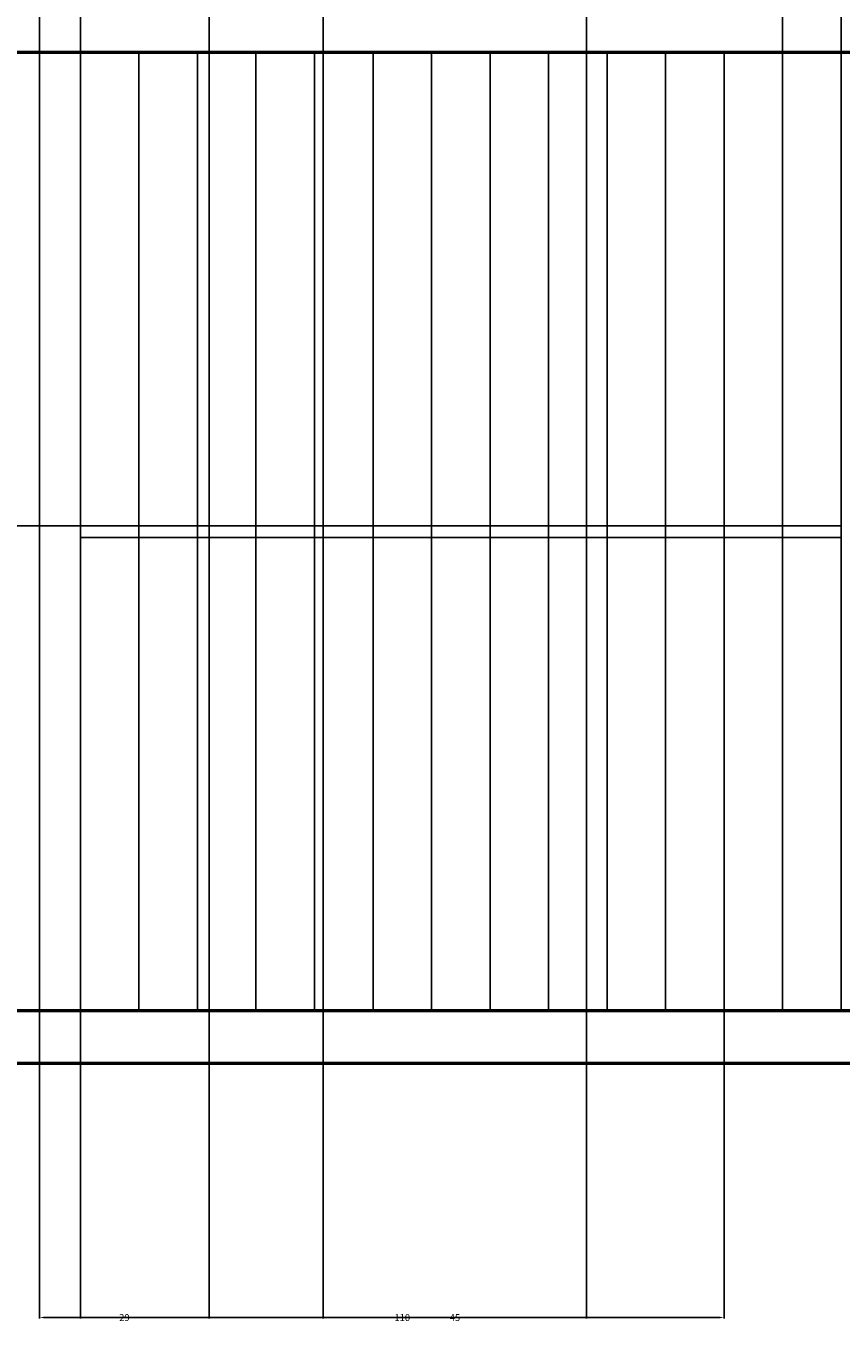
# Model space of a CAD drawing. Units: inches. Extents: x 3506 to 3958, y 1553 to 2506.
# Tile 2 of 16: x 3599 to 3739, y 1553 to 1775. Entities that reach past the tile are written whole.
import ezdxf

# ---------------------------------------------------------------- set-up
doc = ezdxf.new("R2010")
doc.units = ezdxf.units.IN
doc.header["$MEASUREMENT"] = 0
for name, color, linetype, lineweight in [('A-ANNO-DIMS', 2, 'Continuous', 18), ('A-FLOR-STRS', 7, 'Continuous', 25), ('A-WALL', 7, 'Continuous', 50)]:
    doc.layers.add(name, color=color, linetype=linetype, lineweight=lineweight)
doc.layers.add('A-WALL-PATT', color=251, linetype='Continuous', lineweight=13, true_color=0x636466)
doc.styles.get("Standard").update_dxf_attribs({"font": 'arial.ttf'})
doc.dimstyles.get("Standard").update_dxf_attribs({"dimtxt": 1.18, "dimasz": 0.68, "dimexe": 0.18, "dimexo": 0.0625, "dimgap": 0.09, "dimtad": 0, "dimtih": 1, "dimtoh": 1, "dimdec": 1, "dimzin": 0, "dimdsep": 46, "dimlunit": 3, "dimtxsty": 'Standard', "dimcen": 0.09, "dimadec": 0, "dimazin": 0, "dimtfac": 1, "dimtdec": 1, "dimtofl": 0, "dimtmove": 0, "dimatfit": 3, "dimfxl": 1, "dimtolj": 1, "dimtzin": 0, "dimarcsym": 0})

# ---------------------------------------------------------------- blocks, each defined once
blk = doc.blocks.new('*D50')
at = {"layer": 'A-ANNO-DIMS', "color": 0, "lineweight": -2, "transparency": 16777216}
for p, q in [((3608.73, 1606.46), (3608.73, 2505.02)), ((3609.41, 2504.84), (3672.39, 2504.84)), ((3738.05, 2504.84), (3675.07, 2504.84)), ((3738.73, 1606.46), (3738.73, 2505.02))]:
    blk.add_line(p, q, dxfattribs=at)
at = {"layer": 'A-ANNO-DIMS', "color": 0, "transparency": 16777216}
for points in [[(3609.41, 2504.96), (3609.41, 2504.73), (3608.73, 2504.84)], [(3738.05, 2504.96), (3738.05, 2504.73), (3738.73, 2504.84)]]:
    blk.add_solid(points, dxfattribs=at)
at = {"layer": 'Defpoints', "color": 0, "transparency": 16777216}
for p in [(3738.73, 2504.84), (3608.73, 1606.39), (3738.73, 1606.39)]:
    blk.add_point(p, dxfattribs=at)
at = {"layer": 'A-ANNO-DIMS', "color": 0, "transparency": 16777216, "insert": (3673.73, 2504.84), "char_height": 1.18, "attachment_point": 5}
blk.add_mtext('\\A1;130', dxfattribs=at)
blk = doc.blocks.new('*D51')
at = {"layer": 'A-ANNO-DIMS', "color": 0, "lineweight": -2, "transparency": 16777216}
for p, q in [((3608.67, 1689.39), (3508.1, 1689.39)), ((3508.28, 1688.71), (3508.28, 1648.59)), ((3508.28, 1607.07), (3508.28, 1647.2)), ((3608.67, 1606.39), (3508.1, 1606.39))]:
    blk.add_line(p, q, dxfattribs=at)
at = {"layer": 'A-ANNO-DIMS', "color": 0, "transparency": 16777216}
for points in [[(3508.17, 1688.71), (3508.39, 1688.71), (3508.28, 1689.39)], [(3508.17, 1607.07), (3508.39, 1607.07), (3508.28, 1606.39)]]:
    blk.add_solid(points, dxfattribs=at)
at = {"layer": 'Defpoints', "color": 0, "transparency": 16777216}
for p in [(3508.28, 1689.39), (3608.73, 1689.39), (3608.73, 1606.39)]:
    blk.add_point(p, dxfattribs=at)
at = {"layer": 'A-ANNO-DIMS', "color": 0, "transparency": 16777216, "insert": (3508.28, 1647.89), "char_height": 1.18, "attachment_point": 5}
blk.add_mtext('\\A1;83', dxfattribs=at)
blk = doc.blocks.new('*D52')
at = {"layer": 'A-ANNO-DIMS', "color": 0, "lineweight": -2, "transparency": 16777216}
for p, q in [((3560.73, 1606.46), (3560.73, 2505.02)), ((3561.41, 2504.84), (3583.77, 2504.84)), ((3608.05, 2504.84), (3585.69, 2504.84)), ((3608.73, 1606.46), (3608.73, 2505.02))]:
    blk.add_line(p, q, dxfattribs=at)
at = {"layer": 'A-ANNO-DIMS', "color": 0, "transparency": 16777216}
for points in [[(3561.41, 2504.96), (3561.41, 2504.73), (3560.73, 2504.84)], [(3608.05, 2504.96), (3608.05, 2504.73), (3608.73, 2504.84)]]:
    blk.add_solid(points, dxfattribs=at)
at = {"layer": 'Defpoints', "color": 0, "transparency": 16777216}
for p in [(3608.73, 2504.84), (3560.73, 1606.39), (3608.73, 1606.39)]:
    blk.add_point(p, dxfattribs=at)
at = {"layer": 'A-ANNO-DIMS', "color": 0, "transparency": 16777216, "insert": (3584.73, 2504.84), "char_height": 1.18, "attachment_point": 5}
blk.add_mtext('\\A1;48', dxfattribs=at)
blk = doc.blocks.new('*D59')
at = {"layer": 'A-ANNO-DIMS', "color": 0, "lineweight": -2, "transparency": 16777216}
for p, q in [((3728.73, 1689.46), (3728.73, 2505.02)), ((3729.41, 2504.84), (3732.85, 2504.84)), ((3738.05, 2504.84), (3734.61, 2504.84)), ((3738.73, 1689.46), (3738.73, 2505.02))]:
    blk.add_line(p, q, dxfattribs=at)
at = {"layer": 'A-ANNO-DIMS', "color": 0, "transparency": 16777216}
for points in [[(3729.41, 2504.96), (3729.41, 2504.73), (3728.73, 2504.84)], [(3738.05, 2504.96), (3738.05, 2504.73), (3738.73, 2504.84)]]:
    blk.add_solid(points, dxfattribs=at)
at = {"layer": 'Defpoints', "color": 0, "transparency": 16777216}
for p in [(3738.73, 2504.84), (3728.73, 1689.39), (3738.73, 1689.39)]:
    blk.add_point(p, dxfattribs=at)
at = {"layer": 'A-ANNO-DIMS', "color": 0, "transparency": 16777216, "insert": (3733.73, 2504.84), "char_height": 1.18, "attachment_point": 5}
blk.add_mtext('\\A1;10', dxfattribs=at)
blk = doc.blocks.new('*D63')
at = {"layer": 'A-ANNO-DIMS', "color": 0, "lineweight": -2, "transparency": 16777216}
for p, q in [((3869.67, 1800.46), (3508.1, 1800.46)), ((3508.28, 1799.78), (3508.28, 1786.12)), ((3508.28, 1771.07), (3508.28, 1784.74)), ((3869.67, 1770.39), (3508.1, 1770.39))]:
    blk.add_line(p, q, dxfattribs=at)
at = {"layer": 'A-ANNO-DIMS', "color": 0, "transparency": 16777216}
for points in [[(3508.17, 1799.78), (3508.39, 1799.78), (3508.28, 1800.46)], [(3508.17, 1771.07), (3508.39, 1771.07), (3508.28, 1770.39)]]:
    blk.add_solid(points, dxfattribs=at)
at = {"layer": 'Defpoints', "color": 0, "transparency": 16777216}
for p in [(3869.73, 1800.46), (3508.28, 1770.39), (3869.73, 1770.39)]:
    blk.add_point(p, dxfattribs=at)
at = {"layer": 'A-ANNO-DIMS', "color": 0, "transparency": 16777216, "insert": (3508.28, 1785.43), "char_height": 1.18, "attachment_point": 5}
blk.add_mtext('\\A1;30.07', dxfattribs=at)
blk = doc.blocks.new('*D66')
at = {"layer": 'A-ANNO-DIMS', "color": 0, "lineweight": -2, "transparency": 16777216}
for p, q in [((3650.23, 2221.36), (3650.23, 1553.76)), ((3695.23, 2221.36), (3695.23, 1553.76)), ((3650.91, 1553.94), (3671.77, 1553.94)), ((3694.55, 1553.94), (3673.69, 1553.94))]:
    blk.add_line(p, q, dxfattribs=at)
at = {"layer": 'A-ANNO-DIMS', "color": 0, "transparency": 16777216}
for points in [[(3650.91, 1554.06), (3650.91, 1553.83), (3650.23, 1553.94)], [(3694.55, 1554.06), (3694.55, 1553.83), (3695.23, 1553.94)]]:
    blk.add_solid(points, dxfattribs=at)
at = {"layer": 'Defpoints', "color": 0, "transparency": 16777216}
for p in [(3650.23, 2221.43), (3695.23, 2221.43), (3695.23, 1553.94)]:
    blk.add_point(p, dxfattribs=at)
at = {"layer": 'A-ANNO-DIMS', "color": 0, "transparency": 16777216, "insert": (3672.73, 1553.94), "char_height": 1.18, "attachment_point": 5}
blk.add_mtext('\\A1;45', dxfattribs=at)
blk = doc.blocks.new('*D68')
at = {"layer": 'A-ANNO-DIMS', "color": 0, "lineweight": -2, "transparency": 16777216}
for p, q in [((3630.73, 2260.33), (3630.73, 1553.76)), ((3601.73, 2231.33), (3601.73, 1553.76)), ((3602.41, 1553.94), (3615.28, 1553.94)), ((3630.05, 1553.94), (3617.18, 1553.94))]:
    blk.add_line(p, q, dxfattribs=at)
at = {"layer": 'A-ANNO-DIMS', "color": 0, "transparency": 16777216}
for points in [[(3602.41, 1554.06), (3602.41, 1553.83), (3601.73, 1553.94)], [(3630.05, 1554.06), (3630.05, 1553.83), (3630.73, 1553.94)]]:
    blk.add_solid(points, dxfattribs=at)
at = {"layer": 'Defpoints', "color": 0, "transparency": 16777216}
for p in [(3630.73, 2260.39), (3601.73, 2231.39), (3630.73, 1553.94)]:
    blk.add_point(p, dxfattribs=at)
at = {"layer": 'A-ANNO-DIMS', "color": 0, "transparency": 16777216, "insert": (3616.23, 1553.94), "char_height": 1.18, "attachment_point": 5}
blk.add_mtext('\\A1;29', dxfattribs=at)
blk = doc.blocks.new('*D72')
at = {"layer": 'A-ANNO-DIMS', "color": 0, "lineweight": -2, "transparency": 16777216}
for p, q in [((3608.73, 1770.33), (3608.73, 1553.76)), ((3718.73, 1770.33), (3718.73, 1553.76)), ((3609.41, 1553.94), (3662.39, 1553.94)), ((3718.05, 1553.94), (3665.07, 1553.94))]:
    blk.add_line(p, q, dxfattribs=at)
at = {"layer": 'A-ANNO-DIMS', "color": 0, "transparency": 16777216}
for points in [[(3609.41, 1554.06), (3609.41, 1553.83), (3608.73, 1553.94)], [(3718.05, 1554.06), (3718.05, 1553.83), (3718.73, 1553.94)]]:
    blk.add_solid(points, dxfattribs=at)
at = {"layer": 'Defpoints', "color": 0, "transparency": 16777216}
for p in [(3608.73, 1770.39), (3718.73, 1770.39), (3718.73, 1553.94)]:
    blk.add_point(p, dxfattribs=at)
at = {"layer": 'A-ANNO-DIMS', "color": 0, "transparency": 16777216, "insert": (3663.73, 1553.94), "char_height": 1.18, "attachment_point": 5}
blk.add_mtext('\\A1;110', dxfattribs=at)

msp = doc.modelspace()

# ---------------------------------------------------------------- hatches: boundary and pattern name
at = {"layer": 'A-WALL-PATT'}
h = msp.add_hatch(dxfattribs=at)
h.set_pattern_fill('ANSI31', color=256)
h.paths.add_polyline_path([(3911.7302, 2461.3942), (3551.7302, 2461.3942), (3551.7302, 2152.516), (3560.7302, 2152.516), (3560.7302, 2116.516), (3551.7302, 2116.516), (3551.7302, 1920.5711), (3556.2302, 1920.5711), (3560.7302, 1920.5711), (3560.7302, 2000.3942), (3692.7302, 2000.3942), (3692.7302, 1997.3942), (3697.7302, 1997.3942), (3697.7302, 2000.3942), (3771.7302, 2000.3942), (3771.7302, 1997.3942), (3776.7302, 1997.3942), (3776.7302, 1997.7206), (3778.5802, 1997.7206), (3807.5802, 1997.7206), (3807.5802, 1996.4519), (3778.5802, 1996.4519), (3778.5802, 1997.7206), (3776.7302, 1997.7206), (3776.7302, 1997.3942), (3771.7302, 1997.3942), (3771.7302, 2000.3942), (3697.7302, 2000.3942), (3697.7302, 1997.3942), (3692.7302, 1997.3942), (3689.8302, 1997.3942), (3689.8302, 1995.8192), (3653.8302, 1995.8192), (3653.8302, 1997.3942), (3689.8302, 1997.3942), (3692.7302, 1997.3942), (3692.7302, 2000.3942), (3560.7302, 2000.3942), (3560.7302, 1920.5711), (3551.7302, 1920.5711), (3551.7302, 1884.5711), (3551.7302, 1597.3942), (3911.7302, 1597.3942)], flags=17)
h.paths.add_polyline_path([(3596.7302, 2005.3942), (3596.7302, 2057.3035, -0.38730371), (3569.1778, 2085), (3569.15, 2085), (3569.15, 2086.2688), (3598.15, 2086.2688), (3598.15, 2085), (3569.1778, 2085, 0.38730371), (3596.7302, 2057.3035), (3596.7302, 2057.3942), (3601.7302, 2057.3942), (3601.7302, 2055.3942), (3630.7302, 2055.3942), (3630.7302, 2034.3942), (3694.7302, 2034.3942), (3694.7302, 2053.3942), (3699.7302, 2053.3942), (3699.7302, 2005.3942), (3860.7302, 2005.3942), (3860.7302, 2173.3942), (3771.7302, 2173.3942), (3771.7302, 2194.3942), (3776.7302, 2194.3942), (3776.7302, 2178.3942), (3860.7302, 2178.3942), (3860.7302, 2231.3942), (3601.7302, 2231.3942), (3601.7302, 2241.426), (3596.7302, 2241.426), (3596.7302, 2231.3942), (3560.7302, 2231.3942), (3560.7302, 2315.3942), (3596.7302, 2315.3942), (3596.7302, 2312.3942), (3601.7302, 2312.3942), (3601.7302, 2315.3942), (3697.7302, 2315.3942), (3697.7302, 2413.3942), (3692.7302, 2413.3942), (3692.7302, 2320.3942), (3560.7302, 2320.3942), (3560.7302, 2452.3942), (3692.7302, 2452.3942), (3692.7302, 2449.3942), (3697.7302, 2449.3942), (3697.7302, 2452.3942), (3771.7302, 2452.3942), (3771.7302, 2449.3942), (3776.7302, 2449.3942), (3776.7302, 2452.3942), (3860.7302, 2452.3942), (3860.7302, 2437.2075), (3865.2302, 2437.2075), (3865.2302, 2413.2075), (3860.7302, 2413.2075), (3860.7302, 2367.6976), (3865.2302, 2367.6976), (3869.7302, 2367.6976), (3869.7302, 2319.6976), (3860.7302, 2319.6976), (3860.7302, 2211.6248), (3869.7302, 2211.6248), (3869.7302, 2187.6248), (3860.7302, 2187.6248), (3860.7302, 2138.4346), (3865.2302, 2138.4346), (3869.7302, 2138.4346), (3869.7302, 2090.4346), (3860.7302, 2090.4346), (3860.7302, 1985.8449), (3869.7302, 1985.8449), (3869.7302, 1961.8449), (3860.7302, 1961.8449), (3860.7302, 1897.0756), (3865.2302, 1897.0756), (3869.7302, 1897.0756), (3869.7302, 1849.0756), (3860.7302, 1849.0756), (3860.7302, 1847.8112), (3860.7302, 1779.3942), (3596.7302, 1779.3942), (3596.7302, 1831.3942), (3601.7302, 1831.3942), (3601.7302, 1828.3942), (3630.7302, 1828.3942), (3630.7302, 1808.3942), (3691.7302, 1808.3942), (3691.7302, 1815.3942), (3696.7302, 1815.3942), (3696.7302, 1779.3942), (3860.7302, 1779.3942), (3860.7302, 1947.3942), (3771.7302, 1947.3942), (3771.7302, 1968.3942), (3776.7302, 1968.3942), (3776.7302, 1952.3942), (3860.7302, 1952.3942), (3860.7302, 2005.3942)], flags=0)
h.paths.add_polyline_path([(3596.7302, 2038.8546), (3601.7302, 2038.8546), (3601.7302, 2014.8546), (3596.7302, 2014.8546)], flags=0)
h.paths.add_polyline_path([(3564.1688, 2107), (3564.1688, 2167), (3644.1688, 2167), (3644.1688, 2107)], flags=0)
h.paths.add_polyline_path([(3607.0972, 2052.0208), (3620.8472, 2052.0208, -0.41421356), (3621.9931, 2050.875), (3621.9931, 2025.6667, -0.41421356), (3620.8472, 2024.5208), (3607.0972, 2024.5208, -0.41421356), (3605.9514, 2025.6667), (3605.9514, 2050.875, -0.41421356)], flags=0)
h.paths.add_polyline_path([(3578.5688, 2115), (3565.3688, 2115), (3565.3688, 2135.8), (3578.5688, 2135.8), (3578.5688, 2138.2), (3565.3688, 2138.2), (3565.3688, 2159), (3580.5688, 2159), (3580.5688, 2153.8), (3593.7688, 2167), (3593.7688, 2151.8), (3578.5688, 2151.8)], flags=0)
h.paths.add_polyline_path([(3610.9167, 2050.875), (3620.0833, 2050.875, -0.41421356), (3620.8472, 2050.1111), (3620.8472, 2039.6076, -0.41421356), (3620.0833, 2038.8438), (3610.9167, 2038.8438, -0.41421356), (3610.1528, 2039.6076), (3610.1528, 2050.1111, -0.41421356)], flags=0)
h.paths.add_polyline_path([(3610.9167, 2037.6979), (3620.0833, 2037.6979, -0.41421356), (3620.8472, 2036.934), (3620.8472, 2026.4306, -0.41421356), (3620.0833, 2025.6667), (3610.9167, 2025.6667, -0.41421356), (3610.1528, 2026.4306), (3610.1528, 2036.934, -0.41421356)], flags=0)
h.paths.add_polyline_path([(3616.2639, 2044.7639, -1), (3614.7361, 2044.7639, -1)], flags=0)
h.paths.add_polyline_path([(3615.8819, 2044.7639, -1), (3615.1181, 2044.7639, -1)], flags=0)
h.paths.add_polyline_path([(3616.2639, 2031.7778, -1), (3614.7361, 2031.7778, -1)], flags=0)
h.paths.add_polyline_path([(3615.8819, 2031.7778, -1), (3615.1181, 2031.7778, -1)], flags=0)
h.paths.add_polyline_path([(3609.7539, 2021.7868), (3626.9586, 2021.7868), (3626.9586, 2008.8833), (3609.7539, 2008.8833)], flags=0)
h.paths.add_polyline_path([(3610.4708, 2021.07), (3621.2237, 2021.07), (3621.2237, 2009.6002), (3610.4708, 2009.6002)], flags=0)
h.paths.add_polyline_path([(3611.5461, 2019.9947), (3620.1484, 2019.9947), (3620.1484, 2010.6755), (3611.5461, 2010.6755)], flags=0)
h.paths.add_polyline_path([(3621.9405, 2021.07), (3626.2417, 2021.07), (3626.2417, 2009.6002), (3621.9405, 2009.6002)], flags=0)
h.paths.add_polyline_path([(3622.6574, 2020.3531), (3625.5248, 2020.3531), (3625.5248, 2017.4857), (3622.6574, 2017.4857)], flags=0)
h.paths.add_polyline_path([(3622.6574, 2016.7688), (3625.5248, 2016.7688), (3625.5248, 2010.317), (3622.6574, 2010.317)], flags=0)
h.paths.add_polyline_path([(3624.808, 2016.0519), (3624.808, 2013.9013), (3624.0911, 2013.9013), (3624.0911, 2013.1845), (3623.3743, 2013.1845), (3623.3743, 2013.9013), (3623.3743, 2016.0519)], flags=0)
h.paths.add_polyline_path([(3623.0158, 2012.8261), (3625.1664, 2012.8261), (3625.1664, 2012.1092), (3623.0158, 2012.1092)], flags=0)
h.paths.add_polyline_path([(3623.0158, 2011.7508), (3625.1664, 2011.7508), (3625.1664, 2011.0339), (3623.0158, 2011.0339)], flags=0)
h.paths.add_polyline_path([(3650.0591, 2031.8202), (3674.0368, 2031.8202), (3674.0368, 2012.638), (3669.2413, 2012.638), (3669.2413, 2011.8388), (3672.4383, 2011.8388), (3672.4383, 2011.0395), (3651.6576, 2011.0395), (3651.6576, 2011.8388), (3654.8546, 2011.8388), (3654.8546, 2012.638), (3650.0591, 2012.638)], flags=0)
h.paths.add_polyline_path([(3658.0517, 2024.6269, -1), (3651.6576, 2024.6269, -1)], flags=0)
h.paths.add_polyline_path([(3657.2524, 2024.6269, -1), (3652.4569, 2024.6269, -1)], flags=0)
h.paths.add_polyline_path([(3656.4532, 2024.6269, -1), (3653.2561, 2024.6269, -1)], flags=0)
h.paths.add_polyline_path([(3655.6539, 2024.6269, -1), (3654.0554, 2024.6269, -1)], flags=0)
h.paths.add_polyline_path([(3657.2524, 2017.4336, -1), (3652.4569, 2017.4336, -1)], flags=0)
h.paths.add_polyline_path([(3656.4532, 2017.4336, -1), (3653.2561, 2017.4336, -1)], flags=0)
h.paths.add_polyline_path([(3655.6539, 2017.4336, -1), (3654.0554, 2017.4336, -1)], flags=0)
h.paths.add_polyline_path([(3659.6502, 2027.8239), (3664.4457, 2027.8239), (3664.4457, 2015.0358), (3659.6502, 2015.0358)], flags=0)
h.paths.add_polyline_path([(3663.6465, 2027.0247), (3663.6465, 2015.8351), (3660.4494, 2015.8351), (3660.4494, 2027.0247)], flags=0)
h.paths.add_polyline_path([(3562.6688, 1945.5), (3642.6688, 1945.5), (3642.6688, 1885.5), (3562.6688, 1885.5)], flags=0)
h.paths.add_polyline_path([(3671.6391, 2024.6269, -1), (3666.8435, 2024.6269, -1)], flags=0)
h.paths.add_polyline_path([(3670.8398, 2024.6269, -1), (3667.6428, 2024.6269, -1)], flags=0)
h.paths.add_polyline_path([(3672.4383, 2017.4336, -1), (3666.0443, 2017.4336, -1)], flags=0)
h.paths.add_polyline_path([(3670.0405, 2024.6269, -1), (3668.442, 2024.6269, -1)], flags=0)
h.paths.add_polyline_path([(3671.6391, 2017.4336, -1), (3666.8435, 2017.4336, -1)], flags=0)
h.paths.add_polyline_path([(3670.8398, 2017.4336, -1), (3667.6428, 2017.4336, -1)], flags=0)
h.paths.add_polyline_path([(3592.2688, 1945.5), (3592.2688, 1930.3), (3577.0688, 1930.3), (3577.0688, 1893.5), (3563.8688, 1893.5), (3563.8688, 1914.3), (3577.0688, 1914.3), (3577.0688, 1916.7), (3563.8688, 1916.7), (3563.8688, 1937.5), (3579.0688, 1937.5), (3579.0688, 1932.3)], flags=0)
h.paths.add_polyline_path([(3670.0405, 2017.4336, -1), (3668.442, 2017.4336, -1)], flags=0)
h.paths.add_polyline_path([(3596.7302, 2283.3942), (3601.7302, 2283.3942), (3601.7302, 2265.426), (3599.2302, 2265.426), (3599.2302, 2241.426), (3596.7302, 2241.426), (3596.7302, 2265.426)], flags=0)
h.paths.add_polyline_path([(3596.7302, 1810.7006), (3601.7302, 1810.7006), (3601.7302, 1786.7006), (3596.7302, 1786.7006)], flags=0)
h.paths.add_polyline_path([(3560.7302, 1770.3942), (3738.7302, 1770.3942), (3738.7302, 1746.3942), (3738.7302, 1722.3942), (3748.7302, 1722.3942), (3748.7302, 1674.3942), (3560.7302, 1674.3942)], flags=0)
h.paths.add_polyline_path([(3728.7302, 1746.3942), (3728.7302, 1756.0642), (3738.7302, 1746.3942), (3728.7302, 1738.1582), (3728.7302, 1698.3942), (3591.2519, 1698.3942), (3591.2519, 1746.3942)], flags=0)
h.paths.add_polyline_path([(3771.7302, 2399.3942), (3771.7302, 2420.3942), (3776.7302, 2420.3942), (3776.7302, 2404.3942), (3776.7302, 2399.3942)], flags=0)
h.paths.add_polyline_path([(3911.7302, 2461.3942), (3551.7302, 2461.3942), (3551.7302, 2152.516), (3560.7302, 2152.516), (3560.7302, 2116.516), (3551.7302, 2116.516), (3551.7302, 1920.5711), (3560.7302, 1920.5711), (3560.7302, 2000.3942), (3692.7302, 2000.3942), (3692.7302, 1997.3942), (3697.7302, 1997.3942), (3697.7302, 2000.3942), (3771.7302, 2000.3942), (3771.7302, 1997.3942), (3776.7302, 1997.3942), (3776.7302, 1997.7206), (3778.5802, 1997.7206), (3807.5802, 1997.7206), (3807.5802, 1996.4519), (3778.5802, 1996.4519), (3778.5802, 1997.7206), (3776.7302, 1997.7206), (3776.7302, 1997.3942), (3771.7302, 1997.3942), (3771.7302, 2000.3942), (3697.7302, 2000.3942), (3697.7302, 1997.3942), (3692.7302, 1997.3942), (3689.8302, 1997.3942), (3689.8302, 1995.8192), (3653.8302, 1995.8192), (3653.8302, 1997.3942), (3689.8302, 1997.3942), (3692.7302, 1997.3942), (3692.7302, 2000.3942), (3560.7302, 2000.3942), (3560.7302, 1920.5711), (3551.7302, 1920.5711), (3551.7302, 1597.3942), (3911.7302, 1597.3942)], flags=17)

# ---------------------------------------------------------------- linework, layer by layer
at = {"layer": 'A-FLOR-STRS'}
for p, q in [((3608.7302, 1606.3942), (3608.7302, 1770.3942)), ((3608.7302, 1770.3942), (3771.7302, 1770.3942)), ((3618.7302, 1606.3942), (3618.7302, 1770.3942)), ((3628.7302, 1606.3942), (3628.7302, 1770.3942)), ((3638.7302, 1606.3942), (3638.7302, 1770.3942)), ((3648.7302, 1606.3942), (3648.7302, 1770.3942)), ((3658.7302, 1606.3942), (3658.7302, 1770.3942)), ((3668.7302, 1606.3942), (3668.7302, 1770.3942)), ((3678.7302, 1606.3942), (3678.7302, 1770.3942)), ((3688.7302, 1606.3942), (3688.7302, 1770.3942)), ((3698.7302, 1606.3942), (3698.7302, 1770.3942)), ((3708.7302, 1606.3942), (3708.7302, 1770.3942)), ((3718.7302, 1606.3942), (3718.7302, 1770.3942)), ((3608.7302, 1689.3942), (3738.7302, 1689.3942)), ((3608.7302, 1687.3942), (3738.7302, 1687.3942)), ((3728.7302, 1606.3942), (3728.7302, 1689.3942)), ((3738.7302, 1606.3942), (3738.7302, 1689.3942))]:
    msp.add_line(p, q, dxfattribs=at)
at = {"layer": 'A-WALL'}
for p, q in [((3560.7302, 1770.3942), (3771.7302, 1770.3942)), ((3902.7302, 1606.3942), (3560.7302, 1606.3942))]:
    msp.add_line(p, q, dxfattribs=at)
msp.add_lwpolyline([(3551.7302, 2461.3942), (3911.7302, 2461.3942), (3911.7302, 1597.3942), (3551.7302, 1597.3942)], close=True, dxfattribs=at)

# ---------------------------------------------------------------- dimensions: what is measured, and where the dimension line sits
at = {"layer": 'A-ANNO-DIMS'}
for base, p1, p2, picture, middle in [((3608.7302, 2504.8442), (3560.7302, 1606.3942), (3608.7302, 1606.3942), '*D52', (3584.7302, 2504.8442)), ((3738.7302, 2504.8442), (3608.7302, 1606.3942), (3738.7302, 1606.3942), '*D50', (3673.7302, 2504.8442)), ((3738.7302, 2504.8442), (3728.7302, 1689.3942), (3738.7302, 1689.3942), '*D59', (3733.7302, 2504.8442)), ((3630.7302, 1553.9442), (3601.7302, 2231.3942), (3630.7302, 2260.3942), '*D68', (3616.2302, 1553.9442)), ((3695.2302, 1553.9442), (3650.2302, 2221.4254), (3695.2302, 2221.4254), '*D66', (3672.7302, 1553.9442)), ((3718.7302, 1553.9442), (3608.7302, 1770.3942), (3718.7302, 1770.3942), '*D72', (3663.7302, 1553.9442))]:
    dim = msp.add_linear_dim(base=base, p1=p1, p2=p2, dimstyle='Standard', override={"dimdec": 0, "dimlfac": 1, "dimrnd": 0, "dimzin": 0, "dimdsep": 46, "dimlunit": 2}, dxfattribs=at)
    dim.commit()
    dim.dimension.update_dxf_attribs({"geometry": picture, "text_midpoint": middle})
for base, p1, p2, override, picture, middle in [((3508.2802, 1770.3942), (3869.7302, 1800.4628), (3869.7302, 1770.3942), {"dimdec": 2, "dimlfac": 1, "dimrnd": 0, "dimzin": 0, "dimdsep": 46, "dimlunit": 2}, '*D63', (3508.2802, 1785.4285)), ((3508.2802, 1689.3942), (3608.7302, 1606.3942), (3608.7302, 1689.3942), {"dimdec": 0, "dimlfac": 1, "dimrnd": 0, "dimzin": 0, "dimdsep": 46, "dimlunit": 2}, '*D51', (3508.2802, 1647.8942))]:
    dim = msp.add_linear_dim(base=base, p1=p1, p2=p2, angle=90, dimstyle='Standard', override=override, dxfattribs=at)
    dim.commit()
    dim.dimension.update_dxf_attribs({"geometry": picture, "text_midpoint": middle})

doc.saveas('drawing.dxf')
